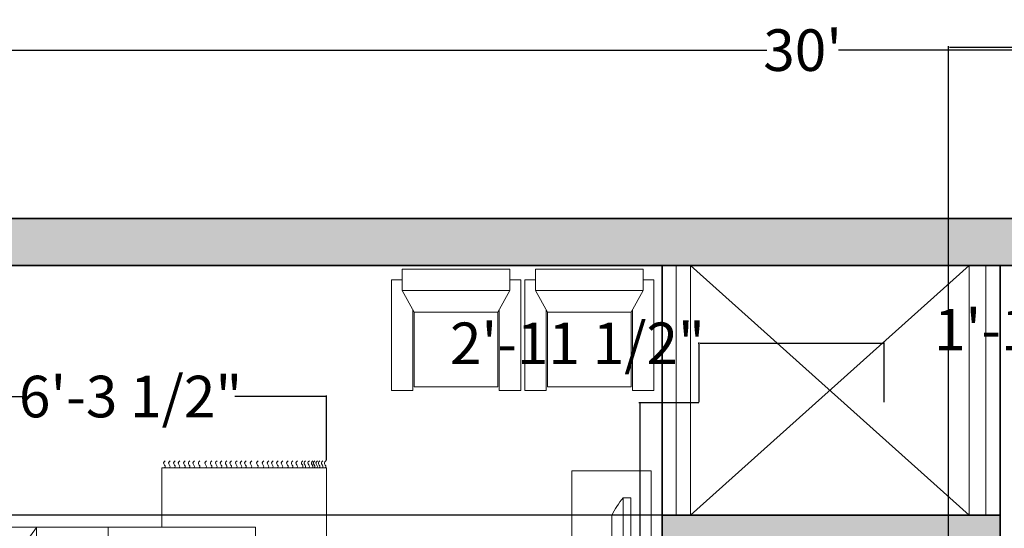
# Model space of a CAD drawing. Units: inches. Extents: x -4737294 to -4736756, y 1716389 to 1717040.
# Tile 21 of 25: x -4737186 to -4736996, y 1716943 to 1717040. Entities that reach past the tile are written whole.
import ezdxf

# ---------------------------------------------------------------- set-up
doc = ezdxf.new("R2010")
doc.units = ezdxf.units.IN
doc.header["$MEASUREMENT"] = 0
for name, color, linetype, lineweight in [('A-ANNO-DIMS', 2, 'Continuous', 18), ('A-FLOR-OPEN', 252, 'Continuous', 18), ('A-WALL-PATT', 244, 'Continuous', 13), ('furniture', 250, 'Continuous', 18), ('walls', 252, 'Continuous', 35)]:
    doc.layers.add(name, color=color, linetype=linetype, lineweight=lineweight)
doc.styles.get("Standard").update_dxf_attribs({"font": 'arial.ttf'})
doc.dimstyles.get("Standard").update_dxf_attribs({"dimtxt": 8, "dimasz": 0.18, "dimexe": 0.18, "dimexo": 0.0625, "dimgap": 0.09, "dimtad": 0, "dimtih": 1, "dimtoh": 1, "dimzin": 0, "dimdsep": 46, "dimlunit": 3, "dimtxsty": 'Standard', "dimcen": 0.09, "dimadec": 0, "dimazin": 0, "dimtfac": 1, "dimtofl": 0, "dimtmove": 0, "dimatfit": 3, "dimfxl": 1, "dimtolj": 1, "dimtzin": 0, "dimarcsym": 0})

# ---------------------------------------------------------------- blocks, each defined once
blk = doc.blocks.new('*D21')
at = {"layer": 'A-ANNO-DIMS', "color": 0, "lineweight": -2, "transparency": 16777216}
for p, q in [((-4737215.14, 1717002.13), (-4737215.14, 1717034.64)), ((-4737214.96, 1717034.46), (-4737042.02, 1717034.46)), ((-4736855.32, 1717034.46), (-4737028.27, 1717034.46)), ((-4736855.14, 1717002.13), (-4736855.14, 1717034.64))]:
    blk.add_line(p, q, dxfattribs=at)
at = {"layer": 'A-ANNO-DIMS', "color": 0, "transparency": 16777216}
for points in [[(-4737214.96, 1717034.49), (-4737214.96, 1717034.43), (-4737215.14, 1717034.46)], [(-4736855.32, 1717034.49), (-4736855.32, 1717034.43), (-4736855.14, 1717034.46)]]:
    blk.add_solid(points, dxfattribs=at)
at = {"layer": 'Defpoints', "color": 0, "transparency": 16777216}
for p in [(-4736855.14, 1717034.46), (-4737215.14, 1717002.06), (-4736855.14, 1717002.06)]:
    blk.add_point(p, dxfattribs=at)
at = {"layer": 'A-ANNO-DIMS', "color": 0, "transparency": 16777216, "insert": (-4737035.14, 1717034.46), "char_height": 8, "attachment_point": 5}
blk.add_mtext("\\A1;30'", dxfattribs=at)
blk = doc.blocks.new('CARPET')
at = {"layer": 'furniture'}
for p, q in [((-51.53, -98.11), (-51.53, -55.12)), ((-51.53, -55.12), (-41.27, -55.12)), ((36, -55.12), (51.55, -55.12)), ((51.55, -55.12), (51.55, -98.11)), ((51.55, -98.11), (-51.53, -98.11))]:
    blk.add_line(p, q, dxfattribs=at)
for points, knots in [([(-53.37, -55.99), (-53.22, -55.8), (-52.9, -55.41), (-52.34, -55.8), (-51.89, -56.08), (-51.65, -55.91), (-51.53, -55.83)], [0, 0, 0, 0, 0.653278, 1.290138, 1.740457, 2.114451, 2.114451, 2.114451, 2.114451]), ([(53.37, -55.99), (53.22, -55.8), (52.9, -55.41), (52.34, -55.8), (51.89, -56.08), (51.65, -55.91), (51.53, -55.83)], [0, 0, 0, 0, 0.653278, 1.290138, 1.740457, 2.114451, 2.114451, 2.114451, 2.114451]), ([(-53.37, -57.26), (-53.22, -57.07), (-52.9, -56.67), (-52.34, -57.07), (-51.89, -57.35), (-51.65, -57.17), (-51.53, -57.1)], [0, 0, 0, 0, 0.653278, 1.290138, 1.740457, 2.114451, 2.114451, 2.114451, 2.114451]), ([(-53.37, -58.59), (-53.22, -58.4), (-52.9, -58.01), (-52.34, -58.4), (-51.89, -58.68), (-51.65, -58.5), (-51.53, -58.43)], [0, 0, 0, 0, 0.653278, 1.290138, 1.740457, 2.114451, 2.114451, 2.114451, 2.114451]), ([(53.37, -57.26), (53.22, -57.07), (52.9, -56.67), (52.34, -57.07), (51.89, -57.35), (51.65, -57.17), (51.53, -57.1)], [0, 0, 0, 0, 0.653278, 1.290138, 1.740457, 2.114451, 2.114451, 2.114451, 2.114451]), ([(53.37, -58.59), (53.22, -58.4), (52.9, -58.01), (52.34, -58.4), (51.89, -58.68), (51.65, -58.5), (51.53, -58.43)], [0, 0, 0, 0, 0.653278, 1.290138, 1.740457, 2.114451, 2.114451, 2.114451, 2.114451]), ([(-53.37, -59.78), (-53.22, -59.58), (-52.9, -59.19), (-52.34, -59.58), (-51.89, -59.86), (-51.65, -59.69), (-51.53, -59.61)], [0, 0, 0, 0, 0.653278, 1.290138, 1.740457, 2.114451, 2.114451, 2.114451, 2.114451]), ([(-53.37, -61.22), (-53.22, -61.02), (-52.9, -60.63), (-52.34, -61.02), (-51.89, -61.3), (-51.65, -61.13), (-51.53, -61.05)], [0, 0, 0, 0, 0.653278, 1.290138, 1.740457, 2.114451, 2.114451, 2.114451, 2.114451]), ([(53.37, -59.78), (53.22, -59.58), (52.9, -59.19), (52.34, -59.58), (51.89, -59.86), (51.65, -59.69), (51.53, -59.61)], [0, 0, 0, 0, 0.653278, 1.290138, 1.740457, 2.114451, 2.114451, 2.114451, 2.114451]), ([(53.37, -61.22), (53.22, -61.02), (52.9, -60.63), (52.34, -61.02), (51.89, -61.3), (51.65, -61.13), (51.53, -61.05)], [0, 0, 0, 0, 0.653278, 1.290138, 1.740457, 2.114451, 2.114451, 2.114451, 2.114451]), ([(-53.37, -62.44), (-53.22, -62.25), (-52.9, -61.86), (-52.34, -62.25), (-51.89, -62.53), (-51.65, -62.36), (-51.53, -62.28)], [0, 0, 0, 0, 0.653278, 1.290138, 1.740457, 2.114451, 2.114451, 2.114451, 2.114451]), ([(-53.37, -63.63), (-53.22, -63.43), (-52.9, -63.04), (-52.34, -63.43), (-51.89, -63.72), (-51.65, -63.54), (-51.53, -63.46)], [0, 0, 0, 0, 0.653278, 1.290138, 1.740457, 2.114451, 2.114451, 2.114451, 2.114451]), ([(53.37, -62.44), (53.22, -62.25), (52.9, -61.86), (52.34, -62.25), (51.89, -62.53), (51.65, -62.36), (51.53, -62.28)], [0, 0, 0, 0, 0.653278, 1.290138, 1.740457, 2.114451, 2.114451, 2.114451, 2.114451]), ([(53.37, -63.63), (53.22, -63.43), (52.9, -63.04), (52.34, -63.43), (51.89, -63.72), (51.65, -63.54), (51.53, -63.46)], [0, 0, 0, 0, 0.653278, 1.290138, 1.740457, 2.114451, 2.114451, 2.114451, 2.114451]), ([(-53.37, -65.07), (-53.22, -64.87), (-52.9, -64.48), (-52.34, -64.87), (-51.89, -65.15), (-51.65, -64.98), (-51.53, -64.9)], [0, 0, 0, 0, 0.653278, 1.290138, 1.740457, 2.114451, 2.114451, 2.114451, 2.114451]), ([(-53.37, -66.76), (-53.22, -66.56), (-52.9, -66.17), (-52.34, -66.56), (-51.89, -66.84), (-51.65, -66.67), (-51.53, -66.59)], [0, 0, 0, 0, 0.653278, 1.290138, 1.740457, 2.114451, 2.114451, 2.114451, 2.114451]), ([(53.37, -65.07), (53.22, -64.87), (52.9, -64.48), (52.34, -64.87), (51.89, -65.15), (51.65, -64.98), (51.53, -64.9)], [0, 0, 0, 0, 0.653278, 1.290138, 1.740457, 2.114451, 2.114451, 2.114451, 2.114451]), ([(53.37, -66.76), (53.22, -66.56), (52.9, -66.17), (52.34, -66.56), (51.89, -66.84), (51.65, -66.67), (51.53, -66.59)], [0, 0, 0, 0, 0.653278, 1.290138, 1.740457, 2.114451, 2.114451, 2.114451, 2.114451]), ([(-53.37, -68.2), (-53.22, -68), (-52.9, -67.61), (-52.34, -68), (-51.89, -68.28), (-51.65, -68.11), (-51.53, -68.03)], [0, 0, 0, 0, 0.653278, 1.290138, 1.740457, 2.114451, 2.114451, 2.114451, 2.114451]), ([(-53.37, -69.53), (-53.22, -69.33), (-52.9, -68.94), (-52.34, -69.33), (-51.89, -69.61), (-51.65, -69.44), (-51.53, -69.36)], [0, 0, 0, 0, 0.653278, 1.290138, 1.740457, 2.114451, 2.114451, 2.114451, 2.114451]), ([(53.37, -68.2), (53.22, -68), (52.9, -67.61), (52.34, -68), (51.89, -68.28), (51.65, -68.11), (51.53, -68.03)], [0, 0, 0, 0, 0.653278, 1.290138, 1.740457, 2.114451, 2.114451, 2.114451, 2.114451]), ([(53.37, -69.53), (53.22, -69.33), (52.9, -68.94), (52.34, -69.33), (51.89, -69.61), (51.65, -69.44), (51.53, -69.36)], [0, 0, 0, 0, 0.653278, 1.290138, 1.740457, 2.114451, 2.114451, 2.114451, 2.114451]), ([(-53.37, -70.79), (-53.22, -70.6), (-52.9, -70.21), (-52.34, -70.6), (-51.89, -70.88), (-51.65, -70.7), (-51.53, -70.63)], [0, 0, 0, 0, 0.653278, 1.290138, 1.740457, 2.114451, 2.114451, 2.114451, 2.114451]), ([(-53.37, -72.12), (-53.22, -71.93), (-52.9, -71.54), (-52.34, -71.93), (-51.89, -72.21), (-51.65, -72.04), (-51.53, -71.96)], [0, 0, 0, 0, 0.653278, 1.290138, 1.740457, 2.114451, 2.114451, 2.114451, 2.114451]), ([(53.37, -70.79), (53.22, -70.6), (52.9, -70.21), (52.34, -70.6), (51.89, -70.88), (51.65, -70.7), (51.53, -70.63)], [0, 0, 0, 0, 0.653278, 1.290138, 1.740457, 2.114451, 2.114451, 2.114451, 2.114451]), ([(53.37, -72.12), (53.22, -71.93), (52.9, -71.54), (52.34, -71.93), (51.89, -72.21), (51.65, -72.04), (51.53, -71.96)], [0, 0, 0, 0, 0.653278, 1.290138, 1.740457, 2.114451, 2.114451, 2.114451, 2.114451]), ([(-53.37, -73.31), (-53.22, -73.11), (-52.9, -72.72), (-52.34, -73.11), (-51.89, -73.4), (-51.65, -73.22), (-51.53, -73.14)], [0, 0, 0, 0, 0.653278, 1.290138, 1.740457, 2.114451, 2.114451, 2.114451, 2.114451]), ([(-53.37, -74.75), (-53.22, -74.55), (-52.9, -74.16), (-52.34, -74.55), (-51.89, -74.83), (-51.65, -74.66), (-51.53, -74.58)], [0, 0, 0, 0, 0.653278, 1.290138, 1.740457, 2.114451, 2.114451, 2.114451, 2.114451]), ([(53.37, -73.31), (53.22, -73.11), (52.9, -72.72), (52.34, -73.11), (51.89, -73.4), (51.65, -73.22), (51.53, -73.14)], [0, 0, 0, 0, 0.653278, 1.290138, 1.740457, 2.114451, 2.114451, 2.114451, 2.114451]), ([(53.37, -74.75), (53.22, -74.55), (52.9, -74.16), (52.34, -74.55), (51.89, -74.83), (51.65, -74.66), (51.53, -74.58)], [0, 0, 0, 0, 0.653278, 1.290138, 1.740457, 2.114451, 2.114451, 2.114451, 2.114451]), ([(-53.37, -75.98), (-53.22, -75.78), (-52.9, -75.39), (-52.34, -75.78), (-51.89, -76.06), (-51.65, -75.89), (-51.53, -75.81)], [0, 0, 0, 0, 0.653278, 1.290138, 1.740457, 2.114451, 2.114451, 2.114451, 2.114451]), ([(-53.37, -77.16), (-53.22, -76.96), (-52.9, -76.57), (-52.34, -76.96), (-51.89, -77.25), (-51.65, -77.07), (-51.53, -76.99)], [0, 0, 0, 0, 0.653278, 1.290138, 1.740457, 2.114451, 2.114451, 2.114451, 2.114451]), ([(53.37, -75.98), (53.22, -75.78), (52.9, -75.39), (52.34, -75.78), (51.89, -76.06), (51.65, -75.89), (51.53, -75.81)], [0, 0, 0, 0, 0.653278, 1.290138, 1.740457, 2.114451, 2.114451, 2.114451, 2.114451]), ([(53.37, -77.16), (53.22, -76.96), (52.9, -76.57), (52.34, -76.96), (51.89, -77.25), (51.65, -77.07), (51.53, -76.99)], [0, 0, 0, 0, 0.653278, 1.290138, 1.740457, 2.114451, 2.114451, 2.114451, 2.114451]), ([(-53.37, -78.6), (-53.22, -78.4), (-52.9, -78.01), (-52.34, -78.4), (-51.89, -78.68), (-51.65, -78.51), (-51.53, -78.43)], [0, 0, 0, 0, 0.653278, 1.290138, 1.740457, 2.114451, 2.114451, 2.114451, 2.114451]), ([(53.37, -78.6), (53.22, -78.4), (52.9, -78.01), (52.34, -78.4), (51.89, -78.68), (51.65, -78.51), (51.53, -78.43)], [0, 0, 0, 0, 0.653278, 1.290138, 1.740457, 2.114451, 2.114451, 2.114451, 2.114451]), ([(-53.37, -80.29), (-53.22, -80.09), (-52.9, -79.7), (-52.34, -80.09), (-51.89, -80.37), (-51.65, -80.2), (-51.53, -80.12)], [0, 0, 0, 0, 0.653278, 1.290138, 1.740457, 2.114451, 2.114451, 2.114451, 2.114451]), ([(-53.37, -81.73), (-53.22, -81.53), (-52.9, -81.14), (-52.34, -81.53), (-51.89, -81.81), (-51.65, -81.64), (-51.53, -81.56)], [0, 0, 0, 0, 0.653278, 1.290138, 1.740457, 2.114451, 2.114451, 2.114451, 2.114451]), ([(53.37, -80.29), (53.22, -80.09), (52.9, -79.7), (52.34, -80.09), (51.89, -80.37), (51.65, -80.2), (51.53, -80.12)], [0, 0, 0, 0, 0.653278, 1.290138, 1.740457, 2.114451, 2.114451, 2.114451, 2.114451]), ([(53.37, -81.73), (53.22, -81.53), (52.9, -81.14), (52.34, -81.53), (51.89, -81.81), (51.65, -81.64), (51.53, -81.56)], [0, 0, 0, 0, 0.653278, 1.290138, 1.740457, 2.114451, 2.114451, 2.114451, 2.114451]), ([(-53.37, -83.06), (-53.22, -82.86), (-52.9, -82.47), (-52.34, -82.86), (-51.89, -83.14), (-51.65, -82.97), (-51.53, -82.89)], [0, 0, 0, 0, 0.653278, 1.290138, 1.740457, 2.114451, 2.114451, 2.114451, 2.114451]), ([(-53.37, -84.18), (-53.22, -83.99), (-52.9, -83.6), (-52.34, -83.99), (-51.89, -84.27), (-51.65, -84.09), (-51.53, -84.02)], [0, 0, 0, 0, 0.653278, 1.290138, 1.740457, 2.114451, 2.114451, 2.114451, 2.114451]), ([(53.37, -83.06), (53.22, -82.86), (52.9, -82.47), (52.34, -82.86), (51.89, -83.14), (51.65, -82.97), (51.53, -82.89)], [0, 0, 0, 0, 0.653278, 1.290138, 1.740457, 2.114451, 2.114451, 2.114451, 2.114451]), ([(53.37, -84.18), (53.22, -83.99), (52.9, -83.6), (52.34, -83.99), (51.89, -84.27), (51.65, -84.09), (51.53, -84.02)], [0, 0, 0, 0, 0.653278, 1.290138, 1.740457, 2.114451, 2.114451, 2.114451, 2.114451]), ([(-53.37, -85.51), (-53.22, -85.32), (-52.9, -84.93), (-52.34, -85.32), (-51.89, -85.6), (-51.65, -85.42), (-51.53, -85.35)], [0, 0, 0, 0, 0.653278, 1.290138, 1.740457, 2.114451, 2.114451, 2.114451, 2.114451]), ([(-53.37, -86.7), (-53.22, -86.5), (-52.9, -86.11), (-52.34, -86.5), (-51.89, -86.78), (-51.65, -86.61), (-51.53, -86.53)], [0, 0, 0, 0, 0.653278, 1.290138, 1.740457, 2.114451, 2.114451, 2.114451, 2.114451]), ([(53.37, -85.51), (53.22, -85.32), (52.9, -84.93), (52.34, -85.32), (51.89, -85.6), (51.65, -85.42), (51.53, -85.35)], [0, 0, 0, 0, 0.653278, 1.290138, 1.740457, 2.114451, 2.114451, 2.114451, 2.114451]), ([(53.37, -86.7), (53.22, -86.5), (52.9, -86.11), (52.34, -86.5), (51.89, -86.78), (51.65, -86.61), (51.53, -86.53)], [0, 0, 0, 0, 0.653278, 1.290138, 1.740457, 2.114451, 2.114451, 2.114451, 2.114451]), ([(-53.37, -88.14), (-53.22, -87.94), (-52.9, -87.55), (-52.34, -87.94), (-51.89, -88.22), (-51.65, -88.05), (-51.53, -87.97)], [0, 0, 0, 0, 0.653278, 1.290138, 1.740457, 2.114451, 2.114451, 2.114451, 2.114451]), ([(-53.37, -89.36), (-53.22, -89.17), (-52.9, -88.78), (-52.34, -89.17), (-51.89, -89.45), (-51.65, -89.28), (-51.53, -89.2)], [0, 0, 0, 0, 0.653278, 1.290138, 1.740457, 2.114451, 2.114451, 2.114451, 2.114451]), ([(53.37, -88.14), (53.22, -87.94), (52.9, -87.55), (52.34, -87.94), (51.89, -88.22), (51.65, -88.05), (51.53, -87.97)], [0, 0, 0, 0, 0.653278, 1.290138, 1.740457, 2.114451, 2.114451, 2.114451, 2.114451]), ([(53.37, -89.36), (53.22, -89.17), (52.9, -88.78), (52.34, -89.17), (51.89, -89.45), (51.65, -89.28), (51.53, -89.2)], [0, 0, 0, 0, 0.653278, 1.290138, 1.740457, 2.114451, 2.114451, 2.114451, 2.114451]), ([(-53.37, -90.55), (-53.22, -90.35), (-52.9, -89.96), (-52.34, -90.35), (-51.89, -90.64), (-51.65, -90.46), (-51.53, -90.38)], [0, 0, 0, 0, 0.653278, 1.290138, 1.740457, 2.114451, 2.114451, 2.114451, 2.114451]), ([(-53.37, -91.99), (-53.22, -91.79), (-52.9, -91.4), (-52.34, -91.79), (-51.89, -92.07), (-51.65, -91.9), (-51.53, -91.82)], [0, 0, 0, 0, 0.653278, 1.290138, 1.740457, 2.114451, 2.114451, 2.114451, 2.114451]), ([(-53.37, -92.69), (-53.22, -92.48), (-52.9, -92.08), (-52.35, -92.49), (-51.89, -92.77), (-51.65, -92.6), (-51.53, -92.52)], [0, 0, 0, 0, 0.663904, 1.307406, 1.757725, 2.131719, 2.131719, 2.131719, 2.131719]), ([(53.37, -90.55), (53.22, -90.35), (52.9, -89.96), (52.34, -90.35), (51.9, -90.63), (51.66, -90.47), (51.55, -90.4)], [0, 0, 0, 0, 0.653278, 1.290138, 1.740457, 2.0926, 2.0926, 2.0926, 2.0926]), ([(53.37, -91.99), (53.22, -91.79), (52.9, -91.4), (52.34, -91.79), (51.9, -92.07), (51.66, -91.91), (51.55, -91.83)], [0, 0, 0, 0, 0.653278, 1.290138, 1.740457, 2.0926, 2.0926, 2.0926, 2.0926]), ([(53.37, -92.69), (53.22, -92.49), (52.9, -92.09), (52.34, -92.49), (51.9, -92.77), (51.66, -92.61), (51.55, -92.53)], [0, 0, 0, 0, 0.656792, 1.295826, 1.746145, 2.098292, 2.098292, 2.098292, 2.098292]), ([(-53.37, -93.61), (-53.22, -93.42), (-52.9, -93.03), (-52.34, -93.42), (-51.89, -93.7), (-51.65, -93.52), (-51.53, -93.45)], [0, 0, 0, 0, 0.653278, 1.290138, 1.740457, 2.114451, 2.114451, 2.114451, 2.114451]), ([(-53.37, -94.55), (-53.22, -94.35), (-52.9, -93.96), (-52.34, -94.35), (-51.89, -94.63), (-51.65, -94.46), (-51.53, -94.38)], [0, 0, 0, 0, 0.653278, 1.290138, 1.740457, 2.114451, 2.114451, 2.114451, 2.114451]), ([(-53.37, -95.05), (-53.22, -94.85), (-52.9, -94.46), (-52.34, -94.85), (-51.89, -95.14), (-51.65, -94.96), (-51.53, -94.88)], [0, 0, 0, 0, 0.653278, 1.290138, 1.740457, 2.114451, 2.114451, 2.114451, 2.114451]), ([(53.37, -93.66), (53.22, -93.46), (52.9, -93.07), (52.34, -93.46), (51.9, -93.74), (51.66, -93.58), (51.55, -93.5)], [0, 0, 0, 0, 0.653278, 1.290138, 1.740457, 2.0926, 2.0926, 2.0926, 2.0926]), ([(53.37, -94.59), (53.22, -94.4), (52.9, -94.01), (52.34, -94.4), (51.9, -94.68), (51.66, -94.51), (51.55, -94.44)], [0, 0, 0, 0, 0.653278, 1.290138, 1.740457, 2.0926, 2.0926, 2.0926, 2.0926]), ([(53.37, -95.1), (53.22, -94.9), (52.9, -94.51), (52.34, -94.9), (51.9, -95.18), (51.66, -95.02), (51.55, -94.94)], [0, 0, 0, 0, 0.653278, 1.290138, 1.740457, 2.0926, 2.0926, 2.0926, 2.0926]), ([(-53.37, -95.73), (-53.22, -95.54), (-52.9, -95.15), (-52.34, -95.54), (-51.89, -95.82), (-51.65, -95.65), (-51.53, -95.57)], [0, 0, 0, 0, 0.653278, 1.290138, 1.740457, 2.114451, 2.114451, 2.114451, 2.114451]), ([(-53.37, -96.38), (-53.22, -96.18), (-52.9, -95.79), (-52.34, -96.18), (-51.89, -96.47), (-51.65, -96.29), (-51.53, -96.21)], [0, 0, 0, 0, 0.653278, 1.290138, 1.740457, 2.114451, 2.114451, 2.114451, 2.114451]), ([(-53.37, -97.17), (-53.22, -96.98), (-52.9, -96.59), (-52.34, -96.98), (-51.89, -97.26), (-51.65, -97.08), (-51.53, -97.01)], [0, 0, 0, 0, 0.653278, 1.290138, 1.740457, 2.114451, 2.114451, 2.114451, 2.114451]), ([(-53.37, -97.99), (-53.22, -97.79), (-52.9, -97.4), (-52.34, -97.79), (-51.89, -98.08), (-51.65, -97.9), (-51.53, -97.82)], [0, 0, 0, 0, 0.653278, 1.290138, 1.740457, 2.114451, 2.114451, 2.114451, 2.114451]), ([(53.37, -95.78), (53.22, -95.58), (52.9, -95.19), (52.34, -95.58), (51.89, -95.86), (51.65, -95.69), (51.53, -95.61)], [0, 0, 0, 0, 0.653278, 1.290138, 1.740457, 2.114451, 2.114451, 2.114451, 2.114451]), ([(53.37, -96.43), (53.22, -96.23), (52.9, -95.84), (52.34, -96.23), (51.89, -96.51), (51.65, -96.34), (51.53, -96.26)], [0, 0, 0, 0, 0.653278, 1.290138, 1.740457, 2.114451, 2.114451, 2.114451, 2.114451]), ([(53.37, -97.22), (53.22, -97.02), (52.9, -96.63), (52.34, -97.02), (51.89, -97.3), (51.65, -97.13), (51.53, -97.05)], [0, 0, 0, 0, 0.653278, 1.290138, 1.740457, 2.114451, 2.114451, 2.114451, 2.114451]), ([(53.37, -97.99), (53.22, -97.79), (52.9, -97.4), (52.34, -97.79), (51.89, -98.08), (51.65, -97.9), (51.53, -97.82)], [0, 0, 0, 0, 0.653278, 1.290138, 1.740457, 2.114451, 2.114451, 2.114451, 2.114451])]:
    blk.add_open_spline(points, degree=3, knots=knots, dxfattribs=at)
blk = doc.blocks.new('A$C58D270C6')
at = {"layer": 'furniture'}
for p, q in [((9.09, 124.13), (9.09, 108.87)), ((1.46, 116.5), (16.73, 116.5)), ((14.97, 94.84), (24.62, 107.92)), ((24.62, 94.93), (24.62, 107.92)), ((42.08, 108), (42.08, 36)), ((14.97, 94.93), (24.62, 94.93)), ((14.97, 94.84), (14.97, 36)), ((16.22, 94.93), (16.22, 36)), ((9.25, 36), (9.25, 20.74)), ((1.62, 28.37), (16.88, 28.37))]:
    blk.add_line(p, q, dxfattribs=at)
for points in [[(18.5, 108), (18.34, 124.13), (-0.16, 124.13), (0, 108)], [(0, 108), (77.91, 108), (77.91, 36), (0, 36)], [(4.09, 94.93), (14.97, 94.93), (14.97, 73.83), (4.09, 73.83)], [(4.09, 65.23), (14.97, 65.23), (14.97, 44.13), (4.09, 44.13)], [(18.65, 19.87), (18.5, 36), (0, 36), (0.16, 19.87)]]:
    blk.add_lwpolyline(points, close=True, dxfattribs=at)
for centre in [(9.09, 116.5), (9.25, 28.37)]:
    blk.add_circle(centre, 5.95, dxfattribs=at)
at = {"layer": 'furniture', "xscale": 0.9312884925094044, "yscale": 0.9312884925094044, "zscale": 0.9312884925094044, "rotation": 90}
blk.add_blockref('CARPET', (3.79, 74.47), dxfattribs=at)
blk = doc.blocks.new('FABRIC SOFA 1S')
at = {"layer": 'furniture'}
for p, q in [((3, 18.12), (34, 18.12)), ((3, 15.12), (3, 18.12)), ((34, 12.12), (34, 18.12)), ((0, -15.12), (0, 15.12)), ((6, 15.12), (0, 15.12)), ((6, -15.12), (6, 15.12)), ((12, 11.75), (6, 15.12)), ((11.33, 12.12), (34, 12.12)), ((6, -15.12), (12, -11.75)), ((11.33, -12.12), (34, -12.12)), ((34, -12.12), (34, -18.12)), ((6, -15.12), (0, -15.12)), ((3, -18.12), (3, -15.12)), ((3, -18.12), (34, -18.12))]:
    blk.add_line(p, q, dxfattribs=at)
blk.add_lwpolyline([(12, -11.75), (12, 11.75), (33, 11.75), (33, -11.75)], close=True, dxfattribs=at)
blk = doc.blocks.new('PLASMA-LARGE')
at = {"layer": 'furniture'}
for p, q in [((-7.26, 0), (7.26, 0)), ((-18.61, -1), (18.61, -1)), ((-8, -1), (-8, -0.74)), ((8, -1), (8, -0.74)), ((-21, -2.5), (21, -2.5)), ((-21, -2.5), (-21, -3.5)), ((21, -2.5), (21, -3.5)), ((-21, -3.5), (21, -3.5)), ((-8, -3.5), (-8, -4.76)), ((8, -3.5), (8, -4.76)), ((-7.26, -5.5), (7.26, -5.5))]:
    blk.add_line(p, q, dxfattribs=at)
for centre, radius, start, end in [((-7.26, -0.74), 0.744, 90, 180), ((7.26, -0.74), 0.744, 0, 90), ((-13.97, -11.05), 11.07, 114.7602, 129.4175), ((13.97, -11.05), 11.07, 50.5825, 65.2398), ((-7.26, -4.76), 0.744, 180, 270), ((7.26, -4.76), 0.744, 270, 0)]:
    blk.add_arc(centre, radius, start, end, dxfattribs=at)
blk = doc.blocks.new('TV-CONSOLE-BEDROOM')
for p, q in [((15.21, 71.77), (0, 71.77)), ((0, 71.77), (0, 0)), ((15.21, 0), (15.21, 71.77)), ((0, 0), (15.21, 0))]:
    blk.add_line(p, q)
at = {"xscale": 1.450199298177205, "yscale": 1.450199298177205, "zscale": 1.450199298177205, "rotation": 90}
blk.add_blockref('PLASMA-LARGE', (6.22, 36.13), dxfattribs=at)
blk = doc.blocks.new('*D28')
at = {"layer": 'A-ANNO-DIMS', "color": 0, "lineweight": -2, "transparency": 16777216}
for p, q in [((-4736969.37, 1716992.37), (-4736973.21, 1716992.37)), ((-4736973.03, 1716992.19), (-4736973.03, 1716984.95)), ((-4736973.03, 1716969.24), (-4736973.03, 1716976.49)), ((-4736969.37, 1716969.06), (-4736973.21, 1716969.06))]:
    blk.add_line(p, q, dxfattribs=at)
at = {"layer": 'A-ANNO-DIMS', "color": 0, "transparency": 16777216}
for points in [[(-4736973.06, 1716992.19), (-4736973, 1716992.19), (-4736973.03, 1716992.37)], [(-4736973.06, 1716969.24), (-4736973, 1716969.24), (-4736973.03, 1716969.06)]]:
    blk.add_solid(points, dxfattribs=at)
at = {"layer": 'Defpoints', "color": 0, "transparency": 16777216}
for p in [(-4736969.31, 1716992.37), (-4736973.03, 1716969.06), (-4736969.31, 1716969.06)]:
    blk.add_point(p, dxfattribs=at)
at = {"layer": 'A-ANNO-DIMS', "color": 0, "transparency": 16777216, "insert": (-4736973.03, 1716980.72), "char_height": 8, "attachment_point": 5}
blk.add_mtext('\\A1;1\'-11 1/2" TYP.', dxfattribs=at)
blk = doc.blocks.new('*D31')
at = {"layer": 'A-ANNO-DIMS', "color": 0, "lineweight": -2, "transparency": 16777216}
for p, q in [((-4737202.03, 1716955.51), (-4737214.51, 1716955.51)), ((-4737214.33, 1716955.33), (-4737214.33, 1716918.54)), ((-4737214.33, 1716873.3), (-4737214.33, 1716910.08)), ((-4737202.03, 1716873.12), (-4737214.51, 1716873.12))]:
    blk.add_line(p, q, dxfattribs=at)
at = {"layer": 'A-ANNO-DIMS', "color": 0, "transparency": 16777216}
for points in [[(-4737214.36, 1716955.33), (-4737214.3, 1716955.33), (-4737214.33, 1716955.51)], [(-4737214.36, 1716873.3), (-4737214.3, 1716873.3), (-4737214.33, 1716873.12)]]:
    blk.add_solid(points, dxfattribs=at)
at = {"layer": 'Defpoints', "color": 0, "transparency": 16777216}
for p in [(-4737214.33, 1716955.51), (-4737201.97, 1716955.51), (-4737201.97, 1716873.12)]:
    blk.add_point(p, dxfattribs=at)
at = {"layer": 'A-ANNO-DIMS', "color": 0, "transparency": 16777216, "insert": (-4737214.33, 1716914.31), "char_height": 8, "attachment_point": 5}
blk.add_mtext('\\A1;BED GROUP 6\'-10 1/2"', dxfattribs=at)
blk = doc.blocks.new('*D32')
at = {"layer": 'A-ANNO-DIMS', "color": 0, "lineweight": -2, "transparency": 16777216}
for p, q in [((-4737201.97, 1716955.57), (-4737201.97, 1716968.04)), ((-4737201.79, 1716967.86), (-4737184.4, 1716967.86)), ((-4737126.87, 1716967.86), (-4737144.27, 1716967.86)), ((-4737126.69, 1716955.57), (-4737126.69, 1716968.04))]:
    blk.add_line(p, q, dxfattribs=at)
at = {"layer": 'A-ANNO-DIMS', "color": 0, "transparency": 16777216}
for points in [[(-4737201.79, 1716967.89), (-4737201.79, 1716967.83), (-4737201.97, 1716967.86)], [(-4737126.87, 1716967.89), (-4737126.87, 1716967.83), (-4737126.69, 1716967.86)]]:
    blk.add_solid(points, dxfattribs=at)
at = {"layer": 'Defpoints', "color": 0, "transparency": 16777216}
for p in [(-4737126.69, 1716967.86), (-4737201.97, 1716955.51), (-4737126.69, 1716955.51)]:
    blk.add_point(p, dxfattribs=at)
at = {"layer": 'A-ANNO-DIMS', "color": 0, "transparency": 16777216, "insert": (-4737164.33, 1716967.86), "char_height": 8, "attachment_point": 5}
blk.add_mtext('\\A1;6\'-3 1/2"', dxfattribs=at)
blk = doc.blocks.new('*D39')
at = {"layer": 'A-ANNO-DIMS', "color": 0, "lineweight": -2, "transparency": 16777216}
for p, q in [((-4737055.1, 1716966.68), (-4737066.63, 1716966.68)), ((-4737066.45, 1716966.5), (-4737066.45, 1716932.89)), ((-4737066.45, 1716890.83), (-4737066.45, 1716924.44)), ((-4737055.1, 1716890.65), (-4737066.63, 1716890.65))]:
    blk.add_line(p, q, dxfattribs=at)
at = {"layer": 'A-ANNO-DIMS', "color": 0, "transparency": 16777216}
for points in [[(-4737066.48, 1716966.5), (-4737066.42, 1716966.5), (-4737066.45, 1716966.68)], [(-4737066.48, 1716890.83), (-4737066.42, 1716890.83), (-4737066.45, 1716890.65)]]:
    blk.add_solid(points, dxfattribs=at)
at = {"layer": 'Defpoints', "color": 0, "transparency": 16777216}
for p in [(-4737055.04, 1716966.68), (-4737066.45, 1716890.65), (-4737055.04, 1716890.65)]:
    blk.add_point(p, dxfattribs=at)
at = {"layer": 'A-ANNO-DIMS', "color": 0, "transparency": 16777216, "insert": (-4737066.45, 1716928.67), "char_height": 8, "attachment_point": 5}
blk.add_mtext('\\A1;WC BLOCK 6\'-4"', dxfattribs=at)
blk = doc.blocks.new('*D40')
at = {"layer": 'A-ANNO-DIMS', "color": 0, "lineweight": -2, "transparency": 16777216}
for p, q in [((-4737055.04, 1716978.09), (-4737055.22, 1716978.09)), ((-4737055.04, 1716966.75), (-4737055.04, 1716978.27)), ((-4737019.67, 1716978.09), (-4737054.86, 1716978.09)), ((-4737019.49, 1716966.75), (-4737019.49, 1716978.27))]:
    blk.add_line(p, q, dxfattribs=at)
at = {"layer": 'A-ANNO-DIMS', "color": 0, "transparency": 16777216}
for points in [[(-4737054.86, 1716978.12), (-4737054.86, 1716978.06), (-4737055.04, 1716978.09)], [(-4737019.67, 1716978.12), (-4737019.67, 1716978.06), (-4737019.49, 1716978.09)]]:
    blk.add_solid(points, dxfattribs=at)
at = {"layer": 'Defpoints', "color": 0, "transparency": 16777216}
for p in [(-4737055.04, 1716978.09), (-4737055.04, 1716966.68), (-4737019.49, 1716966.68)]:
    blk.add_point(p, dxfattribs=at)
at = {"layer": 'A-ANNO-DIMS', "color": 0, "transparency": 16777216, "insert": (-4737078.44, 1716978.09), "char_height": 8, "attachment_point": 5}
blk.add_mtext('\\A1;2\'-11 1/2"', dxfattribs=at)
blk = doc.blocks.new('*D43')
at = {"layer": 'A-ANNO-DIMS', "color": 0, "lineweight": -2, "transparency": 16777216}
for p, q in [((-4736980.34, 1716956.36), (-4736969.46, 1716956.36)), ((-4736969.64, 1716956.18), (-4736969.64, 1716924.7)), ((-4736969.64, 1716884.77), (-4736969.64, 1716916.25)), ((-4736980.34, 1716884.59), (-4736969.46, 1716884.59))]:
    blk.add_line(p, q, dxfattribs=at)
at = {"layer": 'A-ANNO-DIMS', "color": 0, "transparency": 16777216}
for points in [[(-4736969.67, 1716956.18), (-4736969.61, 1716956.18), (-4736969.64, 1716956.36)], [(-4736969.67, 1716884.77), (-4736969.61, 1716884.77), (-4736969.64, 1716884.59)]]:
    blk.add_solid(points, dxfattribs=at)
at = {"layer": 'Defpoints', "color": 0, "transparency": 16777216}
for p in [(-4736980.4, 1716956.36), (-4736969.64, 1716956.36), (-4736980.4, 1716884.59)]:
    blk.add_point(p, dxfattribs=at)
at = {"layer": 'A-ANNO-DIMS', "color": 0, "transparency": 16777216, "insert": (-4736969.64, 1716920.48), "char_height": 8, "attachment_point": 5}
blk.add_mtext('\\A1;TV CONSOLE 6\'-0" TYP.', dxfattribs=at)
blk = doc.blocks.new('*D65')
at = {"layer": 'A-ANNO-DIMS', "color": 0, "lineweight": -2, "transparency": 16777216}
for p, q in [((-4737007.1, 1716596.13), (-4737007.1, 1717035.24)), ((-4737006.92, 1717035.06), (-4736984.27, 1717035.06)), ((-4736984.09, 1716596.13), (-4736984.09, 1717035.24)), ((-4736984.09, 1717035.06), (-4736983.91, 1717035.06))]:
    blk.add_line(p, q, dxfattribs=at)
at = {"layer": 'A-ANNO-DIMS', "color": 0, "transparency": 16777216}
for points in [[(-4737006.92, 1717035.09), (-4737006.92, 1717035.03), (-4737007.1, 1717035.06)], [(-4736984.27, 1717035.09), (-4736984.27, 1717035.03), (-4736984.09, 1717035.06)]]:
    blk.add_solid(points, dxfattribs=at)
at = {"layer": 'Defpoints', "color": 0, "transparency": 16777216}
for p in [(-4736984.09, 1717035.06), (-4737007.1, 1716596.06), (-4736984.09, 1716596.06)]:
    blk.add_point(p, dxfattribs=at)
at = {"layer": 'A-ANNO-DIMS', "color": 0, "transparency": 16777216, "insert": (-4736970.46, 1717035.06), "char_height": 8, "attachment_point": 5}
blk.add_mtext('\\A1;1\'-11"', dxfattribs=at)
blk = doc.blocks.new('*D70')
at = {"layer": 'A-ANNO-DIMS', "color": 0, "lineweight": -2, "transparency": 16777216}
for p, q in [((-4737056.78, 1716993.06), (-4737270.32, 1716993.06)), ((-4737270.14, 1716992.88), (-4737270.14, 1716973.24)), ((-4737270.14, 1716945.24), (-4737270.14, 1716964.89)), ((-4737056.78, 1716945.06), (-4737270.32, 1716945.06))]:
    blk.add_line(p, q, dxfattribs=at)
at = {"layer": 'A-ANNO-DIMS', "color": 0, "transparency": 16777216}
for points in [[(-4737270.17, 1716992.88), (-4737270.11, 1716992.88), (-4737270.14, 1716993.06)], [(-4737270.17, 1716945.24), (-4737270.11, 1716945.24), (-4737270.14, 1716945.06)]]:
    blk.add_solid(points, dxfattribs=at)
at = {"layer": 'Defpoints', "color": 0, "transparency": 16777216}
for p in [(-4737056.72, 1716993.06), (-4737270.14, 1716945.06), (-4737056.72, 1716945.06)]:
    blk.add_point(p, dxfattribs=at)
at = {"layer": 'A-ANNO-DIMS', "color": 0, "transparency": 16777216, "insert": (-4737270.14, 1716969.06), "char_height": 8, "attachment_point": 5}
blk.add_mtext('\\A1;4\'-0"', dxfattribs=at)

msp = doc.modelspace()

# ---------------------------------------------------------------- hatches: boundary and pattern name
at = {"layer": 'A-WALL-PATT'}
h = msp.add_hatch(color=256, dxfattribs=at)
h.dxf.hatch_style = 1
h.paths.add_polyline_path([(-4737206.144, 1716844.565), (-4737110.144, 1716844.565), (-4737110.144, 1716823.907), (-4737105.644, 1716823.907), (-4737105.644, 1716844.565), (-4737098.44, 1716844.565), (-4737098.44, 1716849.065), (-4737206.144, 1716849.065), (-4737206.144, 1716993.065), (-4736864.144, 1716993.065), (-4736864.144, 1716849.065), (-4736963.275, 1716849.065), (-4736994.446, 1716849.065), (-4736997.144, 1716849.065), (-4736997.144, 1716844.565), (-4736864.144, 1716844.565), (-4736864.144, 1716668.565), (-4736934.391, 1716668.565), (-4736934.391, 1716664.065), (-4736864.144, 1716664.065), (-4736864.144, 1716462.065), (-4736855.144, 1716462.065), (-4736855.144, 1717002.065), (-4737215.144, 1717002.065), (-4737215.144, 1716462.065), (-4737206.144, 1716462.065), (-4737206.144, 1716659.065), (-4737062.144, 1716659.065), (-4737062.144, 1716647.493), (-4737057.644, 1716647.493), (-4737057.644, 1716796.565), (-4737071.812, 1716796.565), (-4737071.812, 1716792.065), (-4737070.805, 1716792.065), (-4737062.144, 1716792.065), (-4737062.144, 1716668.065), (-4737206.144, 1716668.065), (-4737206.144, 1716792.065), (-4737093.784, 1716792.065), (-4737093.784, 1716796.565), (-4737206.144, 1716796.565)])
h = msp.add_hatch(color=256, dxfattribs=at)
h.dxf.hatch_style = 1
h.paths.add_polyline_path([(-4737057.644, 1716940.565), (-4737001.644, 1716940.565), (-4737001.644, 1716879.123), (-4736997.144, 1716879.123), (-4736997.144, 1716945.065), (-4737062.144, 1716945.065), (-4737062.144, 1716881.836), (-4737062.144, 1716844.565), (-4737057.644, 1716844.565), (-4736997.144, 1716844.565), (-4736997.144, 1716856.1), (-4737001.644, 1716856.1), (-4737001.644, 1716849.065), (-4737057.644, 1716849.065)])

# ---------------------------------------------------------------- linework, layer by layer
at = {"layer": 'A-FLOR-OPEN'}
for p, q in [((-4737059.428, 1716945.065), (-4737059.428, 1716993.065)), ((-4737056.719, 1716993.065), (-4737056.719, 1716945.065)), ((-4737056.719, 1716993.065), (-4737003.104, 1716945.065)), ((-4737056.719, 1716945.065), (-4737003.104, 1716993.065)), ((-4737003.104, 1716993.065), (-4737003.104, 1716945.065)), ((-4736999.91, 1716945.065), (-4736999.91, 1716993.065))]:
    msp.add_line(p, q, dxfattribs=at)
at = {"layer": 'walls'}
for p, q in [((-4737215.144, 1717002.065), (-4736855.144, 1717002.065)), ((-4737206.144, 1716993.065), (-4736864.144, 1716993.065)), ((-4737062.144, 1716844.565), (-4737062.144, 1716993.065)), ((-4736997.144, 1716844.565), (-4736997.144, 1716993.065)), ((-4737062.144, 1716945.065), (-4736997.144, 1716945.065))]:
    msp.add_line(p, q, dxfattribs=at)

# ---------------------------------------------------------------- block references
at = {"layer": 'furniture', "xscale": 0.685544738852578, "yscale": 0.685544738852578, "zscale": 0.685544738852578, "rotation": 270}
for p in [(-4737101.766, 1716992.333), (-4737076.158, 1716992.333)]:
    msp.add_blockref('FABRIC SOFA 1S', p, dxfattribs=at)
at = {"layer": 'furniture', "xscale": 0.7897983012973059, "yscale": 0.7897983012973059, "zscale": 0.7897983012973059}
msp.add_blockref('A$C58D270C6', (-4737201.848, 1716857.428), dxfattribs=at)
at = {"layer": 'furniture'}
msp.add_blockref('TV-CONSOLE-BEDROOM', (-4737079.496, 1716881.836), dxfattribs=at)

# ---------------------------------------------------------------- dimensions: what is measured, and where the dimension line sits
at = {"layer": 'A-ANNO-DIMS'}
for base, p1, p2, override, picture, middle in [((-4736984.094, 1717035.065), (-4737007.097, 1716596.065), (-4736984.094, 1716596.065), {"dimdec": 1, "dimlfac": 1, "dimrnd": 0, "dimzin": 1, "dimdsep": 46, "dimlunit": 4, "dimfrac": 2}, '*D65', (-4736970.46, 1717035.065)), ((-4736855.144, 1717034.458), (-4737215.144, 1717002.065), (-4736855.144, 1717002.065), {"dimclrd": 0, "dimclre": 0, "dimclrt": 0}, '*D21', (-4737035.144, 1717034.458)), ((-4737126.692, 1716967.863), (-4737201.971, 1716955.505), (-4737126.692, 1716955.505), {"dimdec": 1, "dimlfac": 1, "dimrnd": 0, "dimzin": 1, "dimdsep": 46, "dimlunit": 4, "dimfrac": 2}, '*D32', (-4737164.331, 1716967.863))]:
    dim = msp.add_linear_dim(base=base, p1=p1, p2=p2, dimstyle='Standard', override=override, dxfattribs=at)
    dim.commit()
    dim.dimension.update_dxf_attribs({"geometry": picture, "text_midpoint": middle})
for base, p1, p2, angle, text, picture, middle in [((-4736973.033, 1716969.065), (-4736969.306, 1716992.373), (-4736969.306, 1716969.065), 270, '<> TYP.', '*D28', (-4736973.033, 1716980.719)), ((-4737066.446, 1716890.648), (-4737055.04, 1716966.683), (-4737055.04, 1716890.648), 270, 'WC BLOCK <>', '*D39', (-4737066.446, 1716928.666)), ((-4737214.329, 1716955.505), (-4737201.971, 1716873.12), (-4737201.971, 1716955.505), 90, 'BED GROUP <>', '*D31', (-4737214.329, 1716914.313)), ((-4736969.637, 1716956.359), (-4736980.402, 1716884.592), (-4736980.402, 1716956.359), 90, 'TV CONSOLE <> TYP.', '*D43', (-4736969.637, 1716920.476))]:
    dim = msp.add_linear_dim(base=base, p1=p1, p2=p2, angle=angle, text=text, dimstyle='Standard', override={"dimdec": 1, "dimlfac": 1, "dimrnd": 0, "dimzin": 1, "dimdsep": 46, "dimlunit": 4, "dimfrac": 2}, dxfattribs=at)
    dim.commit()
    dim.dimension.update_dxf_attribs({"geometry": picture, "text_midpoint": middle})
for base, p1, p2, angle, picture, middle in [((-4737270.144, 1716945.065), (-4737056.719, 1716993.065), (-4737056.719, 1716945.065), 90, '*D70', (-4737270.144, 1716969.065)), ((-4737055.04, 1716978.088), (-4737019.494, 1716966.683), (-4737055.04, 1716966.683), 180, '*D40', (-4737078.44, 1716978.088))]:
    dim = msp.add_linear_dim(base=base, p1=p1, p2=p2, angle=angle, dimstyle='Standard', override={"dimdec": 1, "dimlfac": 1, "dimrnd": 0, "dimzin": 1, "dimdsep": 46, "dimlunit": 4, "dimfrac": 2}, dxfattribs=at)
    dim.commit()
    dim.dimension.update_dxf_attribs({"geometry": picture, "text_midpoint": middle})

doc.saveas('drawing.dxf')
